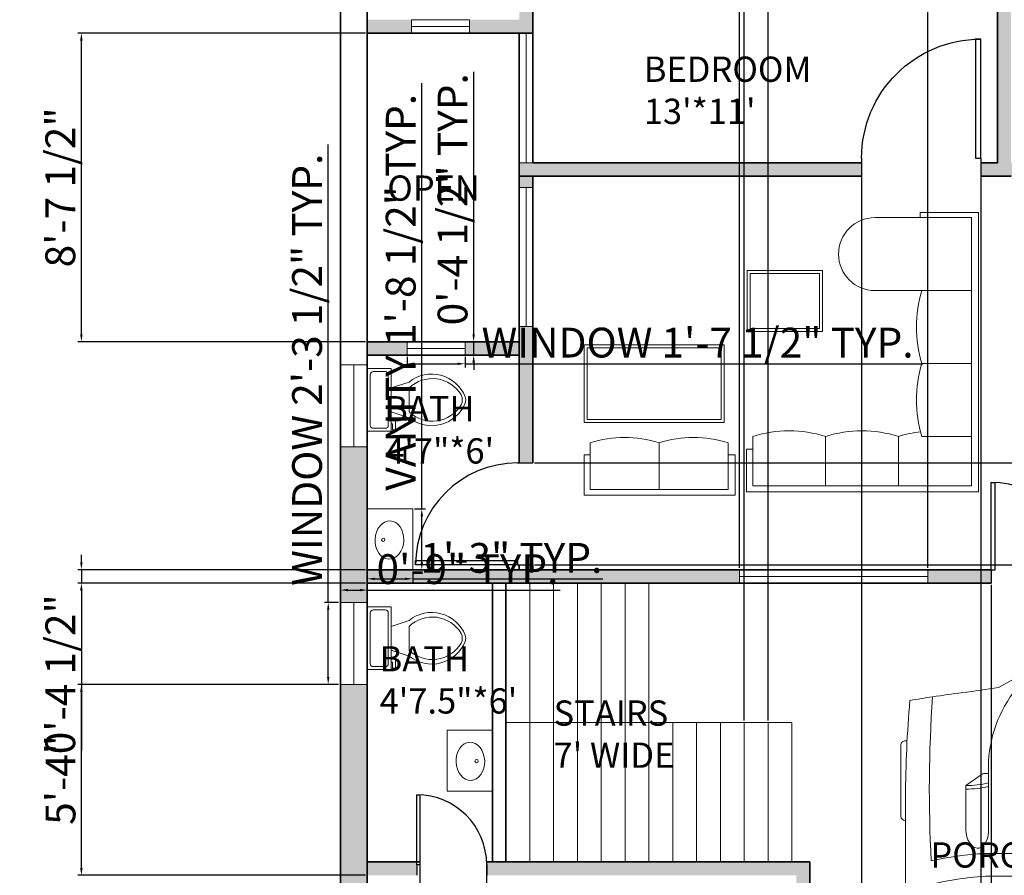
# Model space of a CAD drawing. Units: inches. Extents: x 1698 to 2352, y 1975 to 2732.
# Tile 2 of 4: x 1698 to 2029, y 2234 to 2521. Entities that reach past the tile are written whole.
import ezdxf

# ---------------------------------------------------------------- set-up
doc = ezdxf.new("R2010")
doc.units = ezdxf.units.IN
for name, color, linetype, lineweight in [('A-ANNO-DIMS', 2, 'Continuous', 18), ('A-AREA-IDEN', 7, 'Continuous', 18), ('A-FLOR-FIXT', 231, 'Continuous', 18), ('A-WALL-PATT', 52, 'Continuous', 13), ('car', 171, 'Continuous', 13), ('door', 80, 'Continuous', 25), ('fur', 10, 'Continuous', 18), ('stair', 200, 'Continuous', 18), ('wall', 7, 'Continuous', 35), ('window', 130, 'Continuous', 18)]:
    doc.layers.add(name, color=color, linetype=linetype, lineweight=lineweight)
doc.styles.get("Standard").update_dxf_attribs({"font": 'arial.ttf'})
doc.dimstyles.new('ISO-25', dxfattribs={"dimtxt": 10, "dimasz": 2.5, "dimexe": 1.25, "dimexo": 0.625, "dimtad": 1, "dimdec": 0, "dimlunit": 4, "dimtxsty": 'Standard', "dimcen": 2.5, "dimadec": 0, "dimazin": 0, "dimtfac": 1, "dimtdec": 0, "dimtmove": 0, "dimatfit": 3, "dimfxl": 1, "dimarcsym": 0})

# ---------------------------------------------------------------- blocks, each defined once
blk = doc.blocks.new('*U2')
for p, q in [((0, 0), (0, -6)), ((40, 0), (40, -6))]:
    blk.add_line(p, q)
blk.add_lwpolyline([(0, 0), (0, 40), (1.75, 40), (1.75, 0)], close=True)
blk.add_arc((0, 0), 40, 0, 90)
blk = doc.blocks.new('*U6')
for p, q in [((21.1, 37.41), (21.1, 36.83)), ((46.55, 38.89), (22.35, 38.89)), ((47.8, 37.39), (47.8, 37.41)), ((135.45, 37.07), (135.45, 37.41)), ((136.7, 38.89), (160.9, 38.89)), ((162.15, 37.41), (162.15, 36.77)), ((87.99, 31.87), (74.76, 35.92)), ((134.31, 35.6), (119.29, 31.78)), ((186.47, -33.5), (186.47, 33.5)), ((70.03, 31.54), (86.41, 29.35)), ((188.4, -32.76), (188.4, 32.76)), ((138.42, 29.35), (157.25, 29.35)), ((186.47, 29.35), (167.01, 29.35)), ((164.52, 26.39), (164.52, -26.39)), ((32.27, 11.63), (36.13, 17.17)), ((36.13, 17.17), (50.94, 17.17)), ((32.12, 9.51), (32.12, 11.15)), ((58.92, -10.77), (58.92, 10.77)), ((66.55, -10.53), (66.55, 10.53)), ((186.47, -10.53), (186.47, 10.53)), ((29.77, 9.51), (51.68, 9.51)), ((82.74, 8.5), (82.74, -8.5)), ((3.27, 6.13), (0.1, 0.41)), ((0, 0), (51.68, 0)), ((0.1, -0.41), (3.27, -6.13)), ((29.77, -9.51), (51.68, -9.51)), ((32.12, -9.51), (32.12, -11.15)), ((32.27, -11.63), (36.13, -17.17)), ((36.13, -17.17), (50.94, -17.17)), ((86.41, -29.35), (70.03, -31.54)), ((157.25, -29.35), (138.42, -29.35)), ((167.01, -29.35), (186.47, -29.35)), ((87.99, -31.87), (74.76, -35.92)), ((134.31, -35.6), (119.29, -31.78)), ((21.1, -37.41), (21.1, -36.83)), ((46.55, -38.89), (22.35, -38.89)), ((47.8, -37.39), (47.8, -37.41)), ((135.45, -37.07), (135.45, -37.41)), ((136.7, -38.89), (160.9, -38.89)), ((162.15, -37.41), (162.15, -36.77))]:
    blk.add_line(p, q)
for centre, major_axis, ratio, start_param, end_param in [((41.19, -490.86), (0, 528.23), 0.842304, 0.00281, 0.075598), ((22.35, 37.41), (0, -1.48), 0.842304, 3.141593, 4.712389), ((64.48, -10555.62), (0, 10593.03), 0.842304, -0.013397, 0.002797), ((46.55, 37.41), (0, 1.48), 0.842304, -1.570796, 0), ((136.7, 37.41), (0, -1.48), 0.842304, 3.141593, 4.712389), ((160.9, 37.41), (0, 1.48), 0.842304, -1.570796, 0), ((180.63, 35.84), (0, 2.22), 0.842304, -0.013017, 1.249894), ((64.48, -10556.36), (0, 10595.31), 0.842304, -0.013397, -0.013017), ((183.98, 33.5), (0, -2.96), 0.842304, 1.570796, 3.128196), ((183.98, 32.76), (0, -5.25), 0.842304, 1.570796, 3.128196), ((266.03, -27.52), (0, 313.31), 0.842304, 1.367076, 1.39176), ((64.48, -10555.62), (0, -10591.55), 0.842304, 3.133765, 3.140441), ((135.29, 5.39), (0, 81.77), 0.842304, 1.245306, 1.50788), ((95.79, -3666.35), (0, -3698.24), 0.842304, 3.134049, 3.144098), ((259.18, -27.52), (0, -305.3), 0.842304, 4.528606, 4.561838), ((37.47, -593.96), (0, -623.33), 0.842304, 3.096046, 3.200911), ((134.4, 5.39), (0, -89.78), 0.842304, 4.449482, 4.652344), ((149.6, 2.8), (0, -79.58), 0.842304, 4.372215, 4.640744), ((17.08, 0), (0, 147.02), 0.842304, 4.511394, 4.913384), ((35.91, 0), (0, 147.02), 0.842304, 4.511394, 4.913384), ((167.01, 26.39), (0, 2.96), 0.842304, 0, 1.570796), ((-204.49, 52.4), (0, -250.96), 0.842304, 1.385369, 1.434372), ((13.04, 17.01), (0, 27.42), 0.842304, 4.435146, 4.718221), ((14.2, 17.01), (0, 27.42), 0.842304, 4.435146, 4.718221), ((50.79, 13.34), (6.34, -0.36), 0.603834, -1.395552, 1.581315), ((32.75, 11.15), (0, 0.74), 0.842304, 0.879714, 1.570796), ((29.77, -46.66), (0, 56.17), 0.842304, 0, 0.590319), ((0.62, 0), (0, -0.74), 0.842304, 4.131459, 5.293319), ((29.77, 46.66), (0, 56.17), 0.842304, 2.551274, 3.141593), ((-204.49, -52.4), (0, 250.96), 0.842304, -1.434372, -1.385369), ((13.04, -17.01), (0, -27.42), 0.842304, 1.564964, 1.848039), ((14.2, -17.01), (0, -27.42), 0.842304, 1.564964, 1.848039), ((149.6, -2.8), (0, -79.58), 0.842304, -1.499151, -1.230623), ((32.75, -11.15), (0, -0.74), 0.842304, 4.712389, 5.403472), ((134.4, -5.39), (0, -89.78), 0.842304, -1.510751, -1.307889), ((135.29, -5.39), (0, -81.77), 0.842304, -1.50788, -1.245306), ((259.18, 27.52), (0, 305.3), 0.842304, 1.721348, 1.754579), ((167.01, -26.39), (0, -2.96), 0.842304, 4.712389, 6.283185), ((266.03, 27.52), (0, 313.31), 0.842304, 1.749832, 1.774517), ((37.47, 593.96), (0, -623.33), 0.842304, -0.059319, 0.045547), ((95.79, 3666.35), (0, -3698.24), 0.842304, -0.002505, 0.007544), ((183.98, -32.76), (0, -5.25), 0.842304, 0.013397, 1.570796), ((41.19, 490.86), (0, -528.23), 0.842304, -0.075598, -0.00281), ((64.48, 10555.62), (0, -10591.55), 0.842304, 0.001152, 0.007828), ((183.98, -33.5), (0, 2.96), 0.842304, 3.15499, 4.712389), ((22.35, -37.41), (0, 1.48), 0.842304, 1.570796, 3.141593), ((64.48, 10555.62), (0, 10593.03), 0.842304, 3.138796, 3.15499), ((46.55, -37.41), (0, -1.48), 0.842304, 0, 1.570796), ((136.7, -37.41), (0, -1.48), 0.842304, -1.570796, 0), ((160.9, -37.41), (0, 1.48), 0.842304, 3.141593, 4.712389), ((180.63, -35.84), (0, -2.22), 0.842304, -1.249894, 0.013017), ((64.48, 10556.36), (0, 10595.31), 0.842304, 3.15461, 3.15499)]:
    blk.add_ellipse(centre, major_axis=major_axis, ratio=ratio, start_param=start_param, end_param=end_param)
at = {"extrusion": (0, 0, -1)}
blk.add_ellipse((50.79, -13.34), major_axis=(6.34, 0.36), ratio=0.603834, start_param=-1.395552, end_param=1.581315, dxfattribs=at)
blk = doc.blocks.new('*U4')
for p, q in [((9.5, -6), (9.5, -2)), ((-10, -8.5), (-8, -8.5)), ((-10, -9.5), (-10, -8.5)), ((-7, -9.5), (-10, -9.5)), ((-8, -8.5), (-8, -8)), ((-7, -8), (-7, -9.5)), ((-4, -8), (-6, -14)), ((4, -8), (6, -14)), ((4, -14), (-4, -14))]:
    blk.add_line(p, q)
blk.add_lwpolyline([(10.5, -8), (10.5, 0), (-10.5, 0), (-10.5, -8)], close=True)
for points in [[(-9.5, -2), (-9.5, -6)], [(8.5, -1), (-8.5, -1)], [(-8.5, -7), (8.5, -7)]]:
    blk.add_lwpolyline(points)
for centre, radius, start, end in [((-8.62, -1.88), 0.884, 81.8699, 188.1301), ((8.62, -1.88), 0.884, 351.8699, 98.1301), ((-8.62, -6.12), 0.884, 171.8699, 278.1301), ((8.62, -6.12), 0.884, 261.8699, 8.1301), ((3.52, -21.58), 12.17, 141.4691, 247.9714), ((4.2, -21.82), 11.33, 136.3677, 238.9468), ((-3.52, -21.58), 12.17, 292.0284, 38.5307), ((-4.2, -21.82), 11.33, 301.053, 43.6321), ((0, -27.88), 4, 245.7318, 294.2682), ((0, -29), 4, 254.8605, 285.1395)]:
    blk.add_arc(centre, radius, start, end)
blk = doc.blocks.new('BASIN-VANITY')
blk.add_lwpolyline([(0, 20.39), (15.22, 20.39), (15.22, 0), (0, 0)], close=True)
blk.add_circle((5.32, 10.07), 0.551)
blk.add_ellipse((7.43, 9.98), major_axis=(-0.23, -6.4), ratio=0.75221)
blk = doc.blocks.new('WIN-BATH-19_41')
blk.add_line((0, 2.25), (19.41, 2.25))
blk.add_lwpolyline([(0, 4.5), (19.41, 4.5), (19.41, 0), (0, 0)], close=True)
blk = doc.blocks.new('WIN-BATH-27_526')
blk.add_line((4.5, 27.53), (4.5, 0))
blk.add_lwpolyline([(0, 27.53), (9, 27.53), (9, 0), (0, 0)], close=True)
blk = doc.blocks.new('*D17')
at = {"layer": 'A-ANNO-DIMS', "color": 0, "lineweight": -2, "transparency": 16777216}
for p, q in [((1833.27, 2357.16), (1833.27, 2500.02)), ((1830.84, 2357.16), (1834.52, 2357.16)), ((1833.27, 2339.26), (1833.27, 2354.66)), ((1830.84, 2336.76), (1834.52, 2336.76))]:
    blk.add_line(p, q, dxfattribs=at)
at = {"layer": 'A-ANNO-DIMS', "color": 0, "lineweight": 100, "transparency": 16777216}
for points in [[(1832.85, 2354.66), (1833.69, 2354.66), (1833.27, 2357.16)], [(1832.85, 2339.26), (1833.69, 2339.26), (1833.27, 2336.76)]]:
    blk.add_solid(points, dxfattribs=at)
at = {"layer": 'Defpoints', "color": 0, "lineweight": 100, "transparency": 16777216}
for p in [(1830.21, 2357.16), (1833.27, 2357.16), (1830.21, 2336.76)]:
    blk.add_point(p, dxfattribs=at)
at = {"layer": 'A-ANNO-DIMS', "color": 0, "transparency": 16777216, "insert": (1827.48, 2429.84), "char_height": 10, "attachment_point": 5, "rotation": 90}
blk.add_mtext('VANITY 1\'-8 1/2" TYP.', dxfattribs=at)
blk = doc.blocks.new('*D18')
at = {"layer": 'A-ANNO-DIMS', "color": 0, "lineweight": -2, "transparency": 16777216}
for p, q in [((1814.99, 2336.14), (1814.99, 2332.45)), ((1830.21, 2336.14), (1830.21, 2332.45)), ((1817.49, 2333.7), (1827.71, 2333.7)), ((1830.21, 2333.7), (1893.98, 2333.7))]:
    blk.add_line(p, q, dxfattribs=at)
at = {"layer": 'A-ANNO-DIMS', "color": 0, "lineweight": 100, "transparency": 16777216}
for points in [[(1817.49, 2334.12), (1817.49, 2333.29), (1814.99, 2333.7)], [(1827.71, 2334.12), (1827.71, 2333.29), (1830.21, 2333.7)]]:
    blk.add_solid(points, dxfattribs=at)
at = {"layer": 'Defpoints', "color": 0, "lineweight": 100, "transparency": 16777216}
for p in [(1814.99, 2336.76), (1830.21, 2336.76), (1830.21, 2333.7)]:
    blk.add_point(p, dxfattribs=at)
at = {"layer": 'A-ANNO-DIMS', "color": 0, "transparency": 16777216, "insert": (1863.34, 2339.44), "char_height": 10, "attachment_point": 5}
blk.add_mtext('1\'-3" TYP.', dxfattribs=at)
blk = doc.blocks.new('*D23')
at = {"layer": 'A-ANNO-DIMS', "color": 0, "lineweight": -2, "transparency": 16777216}
for p, q in [((1828.36, 2408.14), (1828.36, 2404.6)), ((1830.86, 2405.85), (1845.27, 2405.85)), ((1847.77, 2408.14), (1847.77, 2404.6)), ((1847.77, 2405.85), (2001.36, 2405.85))]:
    blk.add_line(p, q, dxfattribs=at)
at = {"layer": 'A-ANNO-DIMS', "color": 0, "lineweight": 100, "transparency": 16777216}
for points in [[(1830.86, 2406.27), (1830.86, 2405.43), (1828.36, 2405.85)], [(1845.27, 2406.27), (1845.27, 2405.43), (1847.77, 2405.85)]]:
    blk.add_solid(points, dxfattribs=at)
at = {"layer": 'Defpoints', "color": 0, "lineweight": 100, "transparency": 16777216}
for p in [(1828.36, 2408.76), (1847.77, 2408.76), (1847.77, 2405.85)]:
    blk.add_point(p, dxfattribs=at)
at = {"layer": 'A-ANNO-DIMS', "color": 0, "transparency": 16777216, "insert": (1925.81, 2411.65), "char_height": 10, "attachment_point": 5}
blk.add_mtext('WINDOW 1\'-7 1/2" TYP.', dxfattribs=at)
blk = doc.blocks.new('*D24')
at = {"layer": 'A-ANNO-DIMS', "color": 0, "lineweight": -2, "transparency": 16777216}
for p, q in [((1850.68, 2415.76), (1850.68, 2503.77)), ((1848.39, 2413.26), (1851.93, 2413.26)), ((1850.68, 2408.76), (1850.68, 2413.26)), ((1848.39, 2408.76), (1851.93, 2408.76)), ((1850.68, 2406.26), (1850.68, 2403.76))]:
    blk.add_line(p, q, dxfattribs=at)
at = {"layer": 'A-ANNO-DIMS', "color": 0, "lineweight": 100, "transparency": 16777216}
for points in [[(1850.26, 2415.76), (1851.09, 2415.76), (1850.68, 2413.26)], [(1850.26, 2406.26), (1851.09, 2406.26), (1850.68, 2408.76)]]:
    blk.add_solid(points, dxfattribs=at)
at = {"layer": 'Defpoints', "color": 0, "lineweight": 100, "transparency": 16777216}
for p in [(1847.77, 2413.26), (1850.68, 2413.26), (1847.77, 2408.76)]:
    blk.add_point(p, dxfattribs=at)
at = {"layer": 'A-ANNO-DIMS', "color": 0, "transparency": 16777216, "insert": (1844.88, 2461.02), "char_height": 10, "attachment_point": 5, "rotation": 90}
blk.add_mtext('0\'-4 1/2" TYP.', dxfattribs=at)
blk = doc.blocks.new('*D31')
at = {"layer": 'A-ANNO-DIMS', "color": 0, "lineweight": -2, "transparency": 16777216}
for p, q in [((1801.86, 2325.81), (1801.86, 2479.4)), ((1805.37, 2325.81), (1800.61, 2325.81)), ((1801.86, 2300.78), (1801.86, 2323.31)), ((1805.37, 2298.28), (1800.61, 2298.28))]:
    blk.add_line(p, q, dxfattribs=at)
at = {"layer": 'A-ANNO-DIMS', "color": 0, "lineweight": 100, "transparency": 16777216}
for points in [[(1801.45, 2323.31), (1802.28, 2323.31), (1801.86, 2325.81)], [(1801.45, 2300.78), (1802.28, 2300.78), (1801.86, 2298.28)]]:
    blk.add_solid(points, dxfattribs=at)
at = {"layer": 'Defpoints', "color": 0, "lineweight": 100, "transparency": 16777216}
for p in [(1801.86, 2325.81), (1805.99, 2325.81), (1805.99, 2298.28)]:
    blk.add_point(p, dxfattribs=at)
at = {"layer": 'A-ANNO-DIMS', "color": 0, "transparency": 16777216, "insert": (1796.06, 2403.85), "char_height": 10, "attachment_point": 5, "rotation": 90}
blk.add_mtext('WINDOW 2\'-3 1/2" TYP.', dxfattribs=at)
blk = doc.blocks.new('*D32')
at = {"layer": 'A-ANNO-DIMS', "color": 0, "lineweight": -2, "transparency": 16777216}
for p, q in [((1805.99, 2326.43), (1805.99, 2331.18)), ((1808.49, 2329.93), (1812.49, 2329.93)), ((1814.99, 2326.43), (1814.99, 2331.18)), ((1814.99, 2329.93), (1879.7, 2329.93))]:
    blk.add_line(p, q, dxfattribs=at)
at = {"layer": 'A-ANNO-DIMS', "color": 0, "lineweight": 100, "transparency": 16777216}
for points in [[(1808.49, 2330.35), (1808.49, 2329.52), (1805.99, 2329.93)], [(1812.49, 2330.35), (1812.49, 2329.52), (1814.99, 2329.93)]]:
    blk.add_solid(points, dxfattribs=at)
at = {"layer": 'Defpoints', "color": 0, "lineweight": 100, "transparency": 16777216}
for p in [(1814.99, 2329.93), (1805.99, 2325.81), (1814.99, 2325.81)]:
    blk.add_point(p, dxfattribs=at)
at = {"layer": 'A-ANNO-DIMS', "color": 0, "transparency": 16777216, "insert": (1848.59, 2335.67), "char_height": 10, "attachment_point": 5}
blk.add_mtext('0\'-9" TYP.', dxfattribs=at)
blk = doc.blocks.new('*D35')
at = {"layer": 'A-ANNO-DIMS', "color": 0, "lineweight": -2, "transparency": 16777216}
for p, q in [((1832.59, 2238.14), (1832.59, 1983.28)), ((1855.03, 2238.14), (1855.03, 1983.28)), ((1835.09, 1984.53), (1852.53, 1984.53)), ((1855.03, 1984.53), (1915.49, 1984.53))]:
    blk.add_line(p, q, dxfattribs=at)
at = {"layer": 'A-ANNO-DIMS', "color": 0, "lineweight": 100, "transparency": 16777216}
for points in [[(1835.09, 1984.94), (1835.09, 1984.11), (1832.59, 1984.53)], [(1852.53, 1984.94), (1852.53, 1984.11), (1855.03, 1984.53)]]:
    blk.add_solid(points, dxfattribs=at)
at = {"layer": 'Defpoints', "color": 0, "lineweight": 100, "transparency": 16777216}
for p in [(1832.59, 2238.76), (1855.03, 2238.76), (1855.03, 1984.53)]:
    blk.add_point(p, dxfattribs=at)
at = {"layer": 'A-ANNO-DIMS', "color": 0, "transparency": 16777216, "insert": (1886.51, 1990.32), "char_height": 10, "attachment_point": 5}
blk.add_mtext('1\'-10 1/2"', dxfattribs=at)
blk = doc.blocks.new('*D36')
at = {"layer": 'A-ANNO-DIMS', "color": 0, "lineweight": -2, "transparency": 16777216}
for p, q in [((1941.49, 2286.14), (1941.49, 2651.46)), ((1943.99, 2650.21), (1946.99, 2650.21)), ((1949.49, 2286.14), (1949.49, 2651.46)), ((1949.49, 2650.21), (1979.82, 2650.21))]:
    blk.add_line(p, q, dxfattribs=at)
at = {"layer": 'A-ANNO-DIMS', "color": 0, "lineweight": 100, "transparency": 16777216}
for points in [[(1943.99, 2650.63), (1943.99, 2649.8), (1941.49, 2650.21)], [(1946.99, 2650.63), (1946.99, 2649.8), (1949.49, 2650.21)]]:
    blk.add_solid(points, dxfattribs=at)
at = {"layer": 'Defpoints', "color": 0, "lineweight": 100, "transparency": 16777216}
for p in [(1949.49, 2650.21), (1941.49, 2285.51), (1949.49, 2285.51)]:
    blk.add_point(p, dxfattribs=at)
at = {"layer": 'A-ANNO-DIMS', "color": 0, "transparency": 16777216, "insert": (1965.91, 2655.94), "char_height": 10, "attachment_point": 5}
blk.add_mtext('0\'-8"', dxfattribs=at)
blk = doc.blocks.new('*D37')
at = {"layer": 'A-ANNO-DIMS', "color": 0, "lineweight": -2, "transparency": 16777216}
for p, q in [((2024.3, 2331.64), (2024.3, 1983.28)), ((2083.04, 2331.64), (2083.04, 1983.28)), ((2026.8, 1984.53), (2080.54, 1984.53)), ((2083.04, 1984.53), (2144.84, 1984.53))]:
    blk.add_line(p, q, dxfattribs=at)
at = {"layer": 'A-ANNO-DIMS', "color": 0, "lineweight": 100, "transparency": 16777216}
for points in [[(2026.8, 1984.94), (2026.8, 1984.11), (2024.3, 1984.53)], [(2080.54, 1984.94), (2080.54, 1984.11), (2083.04, 1984.53)]]:
    blk.add_solid(points, dxfattribs=at)
at = {"layer": 'Defpoints', "color": 0, "lineweight": 100, "transparency": 16777216}
for p in [(2024.3, 2332.26), (2083.04, 2332.26), (2083.04, 1984.53)]:
    blk.add_point(p, dxfattribs=at)
at = {"layer": 'A-ANNO-DIMS', "color": 0, "transparency": 16777216, "insert": (2115.19, 1990.32), "char_height": 10, "attachment_point": 5}
blk.add_mtext('4\'-10 1/2"', dxfattribs=at)
blk = doc.blocks.new('*D39')
at = {"layer": 'A-ANNO-DIMS', "color": 0, "lineweight": -2, "transparency": 16777216}
for p, q in [((1980.85, 2472.64), (1980.85, 1983.28)), ((2020.85, 2472.64), (2020.85, 1983.28)), ((1983.35, 1984.53), (2018.35, 1984.53))]:
    blk.add_line(p, q, dxfattribs=at)
at = {"layer": 'A-ANNO-DIMS', "color": 0, "lineweight": 100, "transparency": 16777216}
for points in [[(1983.35, 1984.94), (1983.35, 1984.11), (1980.85, 1984.53)], [(2018.35, 1984.94), (2018.35, 1984.11), (2020.85, 1984.53)]]:
    blk.add_solid(points, dxfattribs=at)
at = {"layer": 'Defpoints', "color": 0, "lineweight": 100, "transparency": 16777216}
for p in [(1980.85, 2473.26), (2020.85, 2473.26), (2020.85, 1984.53)]:
    blk.add_point(p, dxfattribs=at)
at = {"layer": 'A-ANNO-DIMS', "color": 0, "transparency": 16777216, "insert": (2000.85, 1990.26), "char_height": 10, "attachment_point": 5}
blk.add_mtext('3\'-4"', dxfattribs=at)
blk = doc.blocks.new('*D42')
at = {"layer": 'A-ANNO-DIMS', "color": 0, "lineweight": -2, "transparency": 16777216}
for p, q in [((1805.37, 2298.28), (1717.79, 2298.28)), ((1719.04, 2236.76), (1719.04, 2295.78)), ((1814.37, 2234.26), (1717.79, 2234.26))]:
    blk.add_line(p, q, dxfattribs=at)
at = {"layer": 'A-ANNO-DIMS', "color": 0, "lineweight": 100, "transparency": 16777216}
for points in [[(1718.62, 2295.78), (1719.46, 2295.78), (1719.04, 2298.28)], [(1718.62, 2236.76), (1719.46, 2236.76), (1719.04, 2234.26)]]:
    blk.add_solid(points, dxfattribs=at)
at = {"layer": 'Defpoints', "color": 0, "lineweight": 100, "transparency": 16777216}
for p in [(1719.04, 2298.28), (1805.99, 2298.28), (1814.99, 2234.26)]:
    blk.add_point(p, dxfattribs=at)
at = {"layer": 'A-ANNO-DIMS', "color": 0, "transparency": 16777216, "insert": (1713.33, 2266.27), "char_height": 10, "attachment_point": 5, "rotation": 90}
blk.add_mtext('5\'-4"', dxfattribs=at)
blk = doc.blocks.new('*D44')
at = {"layer": 'A-ANNO-DIMS', "color": 0, "lineweight": -2, "transparency": 16777216}
for p, q in [((1719.04, 2339.26), (1719.04, 2341.76)), ((1814.37, 2336.76), (1717.79, 2336.76)), ((1719.04, 2336.76), (1719.04, 2332.26)), ((1814.37, 2332.26), (1717.79, 2332.26)), ((1719.04, 2329.76), (1719.04, 2276.13))]:
    blk.add_line(p, q, dxfattribs=at)
at = {"layer": 'A-ANNO-DIMS', "color": 0, "lineweight": 100, "transparency": 16777216}
for points in [[(1718.62, 2339.26), (1719.46, 2339.26), (1719.04, 2336.76)], [(1718.62, 2329.76), (1719.46, 2329.76), (1719.04, 2332.26)]]:
    blk.add_solid(points, dxfattribs=at)
at = {"layer": 'Defpoints', "color": 0, "lineweight": 100, "transparency": 16777216}
for p in [(1814.99, 2336.76), (1719.04, 2332.26), (1814.99, 2332.26)]:
    blk.add_point(p, dxfattribs=at)
at = {"layer": 'A-ANNO-DIMS', "color": 0, "transparency": 16777216, "insert": (1713.25, 2301.7), "char_height": 10, "attachment_point": 5, "rotation": 90}
blk.add_mtext('0\'-4 1/2"', dxfattribs=at)
blk = doc.blocks.new('*D45')
at = {"layer": 'A-ANNO-DIMS', "color": 0, "lineweight": -2, "transparency": 16777216}
for p, q in [((2342.94, 2372.57), (2342.94, 2410.85)), ((1871.12, 2372.57), (2344.19, 2372.57)), ((2342.94, 2340.87), (2342.94, 2370.07)), ((1871.12, 2338.37), (2344.19, 2338.37))]:
    blk.add_line(p, q, dxfattribs=at)
at = {"layer": 'A-ANNO-DIMS', "color": 0, "lineweight": 100, "transparency": 16777216}
for points in [[(2342.52, 2370.07), (2343.36, 2370.07), (2342.94, 2372.57)], [(2342.52, 2340.87), (2343.36, 2340.87), (2342.94, 2338.37)]]:
    blk.add_solid(points, dxfattribs=at)
at = {"layer": 'Defpoints', "color": 0, "lineweight": 100, "transparency": 16777216}
for p in [(1870.49, 2372.57), (2342.94, 2372.57), (1870.49, 2338.37)]:
    blk.add_point(p, dxfattribs=at)
at = {"layer": 'A-ANNO-DIMS', "color": 0, "transparency": 16777216, "insert": (2337.21, 2392.96), "char_height": 10, "attachment_point": 5, "rotation": 90}
blk.add_mtext('2\'-10"', dxfattribs=at)
blk = doc.blocks.new('*D46')
at = {"layer": 'A-ANNO-DIMS', "color": 0, "lineweight": -2, "transparency": 16777216}
for p, q in [((1814.37, 2516.76), (1717.79, 2516.76)), ((1719.04, 2415.76), (1719.04, 2514.26)), ((1814.37, 2413.26), (1717.79, 2413.26))]:
    blk.add_line(p, q, dxfattribs=at)
at = {"layer": 'A-ANNO-DIMS', "color": 0, "lineweight": 100, "transparency": 16777216}
for points in [[(1718.62, 2514.26), (1719.46, 2514.26), (1719.04, 2516.76)], [(1718.62, 2415.76), (1719.46, 2415.76), (1719.04, 2413.26)]]:
    blk.add_solid(points, dxfattribs=at)
at = {"layer": 'Defpoints', "color": 0, "lineweight": 100, "transparency": 16777216}
for p in [(1719.04, 2516.76), (1814.99, 2516.76), (1814.99, 2413.26)]:
    blk.add_point(p, dxfattribs=at)
at = {"layer": 'A-ANNO-DIMS', "color": 0, "transparency": 16777216, "insert": (1713.25, 2465.01), "char_height": 10, "attachment_point": 5, "rotation": 90}
blk.add_mtext('8\'-7 1/2"', dxfattribs=at)
blk = doc.blocks.new('*D50')
at = {"layer": 'A-ANNO-DIMS', "color": 0, "lineweight": -2, "transparency": 16777216}
for p, q in [((1939.87, 2337.39), (1939.87, 2651.46)), ((1942.37, 2650.21), (2000.54, 2650.21)), ((2003.04, 2337.39), (2003.04, 2651.46))]:
    blk.add_line(p, q, dxfattribs=at)
at = {"layer": 'A-ANNO-DIMS', "color": 0, "lineweight": 100, "transparency": 16777216}
for points in [[(1942.37, 2650.63), (1942.37, 2649.8), (1939.87, 2650.21)], [(2000.54, 2650.63), (2000.54, 2649.8), (2003.04, 2650.21)]]:
    blk.add_solid(points, dxfattribs=at)
at = {"layer": 'Defpoints', "color": 0, "lineweight": 100, "transparency": 16777216}
for p in [(2003.04, 2650.21), (1939.87, 2336.76), (2003.04, 2336.76)]:
    blk.add_point(p, dxfattribs=at)
at = {"layer": 'A-ANNO-DIMS', "color": 0, "transparency": 16777216, "insert": (1971.45, 2655.95), "char_height": 10, "attachment_point": 5}
blk.add_mtext('5\'-3"', dxfattribs=at)

msp = doc.modelspace()

# ---------------------------------------------------------------- hatches: boundary and pattern name
at = {"layer": 'A-WALL-PATT'}
h = msp.add_hatch(color=256, dxfattribs=at)
h.dxf.hatch_style = 1
h.paths.add_polyline_path([(1910.52, 2614.26), (1805.99, 2614.26), (1805.99, 2549.47), (1814.99, 2549.47), (1814.99, 2605.26), (1910.52, 2605.26)])
h.paths.add_polyline_path([(2084.19, 2614.26), (1972.89, 2614.26), (1972.89, 2605.26), (2026.49, 2605.26), (2084.19, 2605.26)])
h.paths.add_polyline_path([(2255.99, 2614.26), (2146.56, 2614.26), (2146.56, 2605.26), (2148.21, 2605.26), (2186.99, 2605.26), (2246.99, 2605.26), (2246.99, 2546.53), (2255.99, 2546.53)])
h.paths.add_polyline_path([(2191.49, 2605.26), (2186.99, 2605.26), (2186.99, 2595.02), (2191.49, 2595.02)], flags=17)
h.paths.add_polyline_path([(2191.49, 2563.28), (2186.99, 2563.28), (2186.99, 2510.76), (2191.49, 2510.76)])
h.paths.add_polyline_path([(2246.99, 2515.26), (2191.49, 2515.26), (2191.49, 2510.76), (2246.99, 2510.76)])
h.paths.add_polyline_path([(2030.99, 2605.26), (2026.49, 2605.26), (2026.49, 2473.26), (2020.85, 2473.26), (2020.85, 2468.76), (2030.99, 2468.76)])
h.paths.add_polyline_path([(1980.85, 2473.26), (1870.49, 2473.26), (1865.99, 2473.26), (1865.99, 2468.76), (1980.85, 2468.76)])
h.paths.add_polyline_path([(1828.36, 2413.26), (1814.99, 2413.26), (1814.99, 2408.76), (1828.36, 2408.76)])
h.paths.add_polyline_path([(1865.99, 2413.26), (1847.77, 2413.26), (1847.77, 2408.76), (1865.99, 2408.76)])
h.paths.add_polyline_path([(1870.49, 2418.36), (1865.99, 2418.36), (1865.99, 2372.57), (1870.49, 2372.57)])
h.paths.add_polyline_path([(2036.32, 2473.26), (2030.99, 2473.26), (2030.99, 2468.76), (2036.32, 2468.76)])
h.paths.add_polyline_path([(2191.49, 2473.26), (2186.99, 2473.26), (2076.32, 2473.26), (2076.32, 2468.76), (2191.49, 2468.76)])
h.paths.add_polyline_path([(2246.99, 2471.76), (2191.49, 2471.76), (2191.49, 2468.76), (2246.99, 2468.76)])
h.paths.add_polyline_path([(2255.99, 2406.37), (2246.99, 2406.37), (2246.99, 2404.25), (2246.99, 2336.76), (2246.99, 2083.26), (2127.92, 2083.26), (2127.92, 2074.26), (2255.99, 2074.26)])
h.paths.add_polyline_path([(2110.49, 2336.76), (2083.04, 2336.76), (2083.04, 2336.67), (2083.04, 2332.26), (2110.49, 2332.26)])
h.paths.add_polyline_path([(2024.3, 2336.76), (2003.04, 2336.76), (2003.04, 2332.26), (2024.3, 2332.26)])
h.paths.add_polyline_path([(2246.99, 2164.26), (2216.76, 2164.26), (2216.76, 2155.26), (2246.99, 2155.26)], flags=17)
h.paths.add_polyline_path([(1958.99, 2083.26), (1927.89, 2083.26), (1927.89, 2074.26), (1958.99, 2074.26)])
h.paths.add_polyline_path([(1963.49, 2185.34), (1958.99, 2185.34), (1958.99, 2083.26), (1963.49, 2083.26)])
h.paths.add_polyline_path([(1963.49, 2238.76), (1855.03, 2238.76, -0.010403), (1855.05, 2237.79), (1855.05, 2234.26), (1958.99, 2234.26), (1958.99, 2225.34), (1963.49, 2225.34)])
h.paths.add_polyline_path([(1831.56, 2237.79), (1831.56, 2238.76), (1814.99, 2238.76), (1814.99, 2234.26), (1831.56, 2234.26)])
h.paths.add_polyline_path([(1939.87, 2336.76), (1814.99, 2336.76), (1814.99, 2332.26), (1856.99, 2332.26), (1939.87, 2332.26)])
h.paths.add_polyline_path([(1814.99, 2377.93), (1805.99, 2377.93), (1805.99, 2325.81), (1814.99, 2325.81)])
h.paths.add_polyline_path([(1829.84, 2521.26), (1814.99, 2521.26), (1814.99, 2516.76), (1829.84, 2516.76)])
h.paths.add_polyline_path([(2255.99, 2471.76), (2246.99, 2471.76), (2246.99, 2438.09), (2255.99, 2438.09)])
h = msp.add_hatch(color=256, dxfattribs=at)
h.dxf.hatch_style = 1
h.paths.add_polyline_path([(1870.49, 2565.42), (1865.99, 2565.42), (1865.99, 2521.26), (1849.25, 2521.26), (1849.25, 2516.76), (1870.49, 2516.76)])
h.paths.add_polyline_path([(1870.49, 2605.26), (1865.99, 2605.26), (1865.99, 2598.8), (1870.49, 2598.8)])
h.paths.add_polyline_path([(2246.99, 2336.76), (2147.99, 2336.76), (2147.99, 2360.76), (2147.99, 2418.65), (2143.49, 2418.65), (2143.49, 2332.26), (2246.99, 2332.26)])
h.paths.add_polyline_path([(2143.49, 2336.76), (2110.49, 2336.76), (2110.49, 2325.07), (2114.99, 2325.07), (2114.99, 2332.26), (2143.49, 2332.26)])
h.paths.add_polyline_path([(2114.99, 2285.07), (2110.49, 2285.07), (2110.49, 2155.26), (2141.76, 2155.26), (2141.76, 2164.26), (2114.99, 2164.26)])
h.paths.add_polyline_path([(1814.99, 2298.28), (1805.99, 2298.28), (1805.99, 2074.26), (1852.89, 2074.26), (1852.89, 2083.26), (1814.99, 2083.26)])
h = msp.add_hatch(color=256, dxfattribs=at)
h.dxf.hatch_style = 1
h.paths.add_polyline_path([(1870.49, 2468.76), (1865.99, 2468.76), (1865.99, 2464.98), (1870.49, 2464.98)])

# ---------------------------------------------------------------- linework, layer by layer
at = {"layer": 'fur'}
for p, q in [((2020.07, 2456.59), (2000.5, 2456.59)), ((2000.5, 2456.59), (2000.5, 2454.86)), ((2020.07, 2377.16), (2020.07, 2456.59)), ((1985.35, 2454.86), (2001.1, 2454.86)), ((2017.68, 2454.86), (2001.1, 2454.86)), ((2017.68, 2430.4), (2017.68, 2454.86)), ((2001.1, 2430.4), (1985.35, 2430.4)), ((2017.68, 2430.4), (2001.1, 2430.4)), ((2001.1, 2430.4), (2017.68, 2430.4)), ((2017.68, 2405.94), (2017.68, 2430.4)), ((2017.68, 2405.94), (2001.1, 2405.94)), ((2001.1, 2405.94), (2017.68, 2405.94)), ((2017.68, 2381.48), (2017.68, 2405.94)), ((1912.9, 2379.34), (1912.9, 2363.66)), ((1968.77, 2381.48), (1968.77, 2364.9)), ((1968.77, 2381.48), (1968.77, 2364.9)), ((1993.23, 2364.9), (1993.23, 2381.48)), ((1993.23, 2381.48), (1993.23, 2364.9)), ((2001.1, 2381.48), (2017.68, 2381.48)), ((2017.68, 2364.9), (2017.68, 2381.48)), ((1944.31, 2377.16), (1942.24, 2377.16)), ((1942.24, 2377.16), (1942.24, 2362.91)), ((1944.31, 2377.16), (1944.31, 2377.16)), ((2020.07, 2362.91), (2020.07, 2377.16)), ((1889.75, 2375.26), (1887.8, 2375.26)), ((1887.8, 2375.26), (1887.8, 2361.77)), ((1889.75, 2375.26), (1889.75, 2375.26)), ((1938.41, 2375.26), (1936.04, 2375.26)), ((1938.41, 2361.77), (1938.41, 2375.26)), ((1942.24, 2362.91), (1995.74, 2362.91)), ((1968.77, 2364.9), (1993.23, 2364.9)), ((1993.23, 2364.9), (2017.68, 2364.9)), ((1995.74, 2362.91), (2020.07, 2362.91)), ((1887.8, 2361.77), (1938.41, 2361.77))]:
    msp.add_line(p, q, dxfattribs=at)
for points in [[(1942.41, 2437.12), (1967.78, 2437.12), (1967.78, 2416.66), (1942.41, 2416.66)], [(1943.41, 2436.12), (1966.78, 2436.12), (1966.78, 2417.66), (1943.41, 2417.66)], [(1887.74, 2386.16), (1934.69, 2386.16), (1934.69, 2412.22), (1887.74, 2412.22)], [(1888.74, 2387.16), (1933.69, 2387.16), (1933.69, 2411.22), (1888.74, 2411.22)]]:
    msp.add_lwpolyline(points, close=True, dxfattribs=at)
for points in [[(1936.04, 2379.34), (1936.04, 2363.66), (1889.75, 2363.66), (1889.75, 2379.34)], [(1993.23, 2381.48), (1993.23, 2364.9), (1944.31, 2364.9), (1944.31, 2381.48)]]:
    msp.add_lwpolyline(points, dxfattribs=at)
for centre, radius, start, end in [((1985.35, 2442.63), 12.23, 90, 270), ((2040.26, 2418.17), 41.02, 162.6553, 197.3447), ((2040.26, 2393.71), 41.02, 162.6553, 197.3447), ((1956.54, 2342.32), 41.02, 72.6553, 107.3447), ((1981, 2342.32), 41.02, 72.6553, 107.3447), ((1981, 2342.32), 41.02, 72.6553, 107.3447), ((2005.45, 2342.32), 41.02, 96.7335, 107.3447), ((1901.32, 2342.3), 38.81, 72.6553, 107.3447), ((1924.47, 2342.3), 38.81, 72.6553, 107.3447)]:
    msp.add_arc(centre, radius, start, end, dxfattribs=at)
at = {"layer": 'stair'}
for p, q in [((1861.49, 2285.51), (1861.49, 2332.26)), ((1869.49, 2332.26), (1869.49, 2238.76)), ((1877.49, 2332.26), (1877.49, 2238.76)), ((1885.49, 2332.26), (1885.49, 2238.76)), ((1893.49, 2332.26), (1893.49, 2238.76)), ((1901.49, 2332.26), (1901.49, 2238.76)), ((1909.49, 2332.26), (1909.49, 2238.76)), ((1861.49, 2285.51), (1956.82, 2285.51)), ((1917.49, 2285.51), (1917.49, 2238.76)), ((1925.49, 2285.51), (1925.49, 2238.76)), ((1933.49, 2285.51), (1933.49, 2238.76)), ((1941.49, 2285.51), (1941.49, 2238.76)), ((1949.49, 2285.51), (1949.49, 2238.76)), ((1957.49, 2285.51), (1956.82, 2285.51)), ((1957.49, 2285.51), (1957.49, 2238.76))]:
    msp.add_line(p, q, dxfattribs=at)
at = {"layer": 'wall'}
for p, q in [((2026.49, 2605.26), (2026.49, 2473.26)), ((1870.49, 2516.76), (1870.49, 2565.42)), ((1814.99, 2516.76), (1870.49, 2516.76)), ((1814.99, 2516.76), (1814.99, 2416.96)), ((1865.99, 2468.76), (1865.99, 2516.76)), ((1870.49, 2473.26), (1870.49, 2516.76)), ((1980.85, 2473.26), (1870.49, 2473.26)), ((2026.49, 2473.26), (2020.85, 2473.26)), ((1865.99, 2468.76), (1865.99, 2372.57)), ((1980.85, 2468.76), (1865.99, 2468.76)), ((1870.49, 2468.76), (1870.49, 2372.57)), ((2030.99, 2468.76), (2020.85, 2468.76)), ((1814.99, 2416.96), (1814.99, 2413.26)), ((1814.99, 2413.26), (1865.99, 2413.26)), ((1814.99, 2336.76), (1814.99, 2408.76)), ((1814.99, 2408.76), (1865.99, 2408.76)), ((2003.04, 2336.76), (1814.99, 2336.76)), ((1865.99, 2338.37), (1865.99, 2336.76)), ((1870.49, 2338.37), (1870.49, 2336.76)), ((2003.04, 2336.76), (2024.3, 2336.76)), ((1814.99, 2332.26), (1856.99, 2332.26)), ((2003.04, 2332.26), (1814.99, 2332.26)), ((1856.99, 2332.26), (1856.99, 2238.76)), ((1861.49, 2332.26), (1861.49, 2238.76)), ((2003.04, 2332.26), (2024.3, 2332.26)), ((1832.59, 2238.76), (1814.99, 2238.76)), ((1963.49, 2238.76), (1855.03, 2238.76)), ((1963.49, 2225.34), (1963.49, 2238.76))]:
    msp.add_line(p, q, dxfattribs=at)
for points in [[(2127.92, 2074.26), (2255.99, 2074.26), (2255.99, 2614.26), (1805.99, 2614.26), (1805.99, 2074.26), (1958.99, 2074.26)], [(2127.92, 2083.26), (2246.99, 2083.26), (2246.99, 2605.26), (1814.99, 2605.26), (1814.99, 2516.76)], [(1814.99, 2413.26), (1814.99, 2083.26), (1976.89, 2083.26)]]:
    msp.add_lwpolyline(points, dxfattribs=at)
at = {"layer": 'window'}
for p, q in [((1868.24, 2516.76), (1868.24, 2473.26)), ((1868.24, 2418.36), (1868.24, 2464.98)), ((1939.87, 2334.51), (2003.04, 2334.51))]:
    msp.add_line(p, q, dxfattribs=at)
for points in [[(1865.99, 2516.76), (1870.49, 2516.76), (1870.49, 2473.26), (1865.99, 2473.26)], [(1865.99, 2418.36), (1870.49, 2418.36), (1870.49, 2464.98), (1865.99, 2464.98)], [(1939.87, 2336.76), (2003.04, 2336.76), (2003.04, 2332.26), (1939.87, 2332.26)]]:
    msp.add_lwpolyline(points, close=True, dxfattribs=at)

# ---------------------------------------------------------------- block references
at = {"layer": 'A-FLOR-FIXT', "rotation": 90}
for p in [(1814.99, 2393.73), (1814.99, 2313.77)]:
    msp.add_blockref('*U4', p, dxfattribs=at)
at = {"layer": 'A-FLOR-FIXT'}
msp.add_blockref('BASIN-VANITY', (1814.99, 2336.76), dxfattribs=at)
at = {"layer": 'A-FLOR-FIXT', "extrusion": (0, 0, -1), "zscale": -1}
msp.add_blockref('BASIN-VANITY', (-1856.99, 2262.5), dxfattribs=at)
at = {"layer": 'car', "rotation": 270}
msp.add_blockref('*U6', (2032.95, 2300.49), dxfattribs=at)
at = {"layer": 'door', "xscale": -1}
msp.add_blockref('*U2', (2020.85, 2474.76), dxfattribs=at)
at = {"layer": 'door', "xscale": 0.8550076532473024, "yscale": 0.8550076532473024, "zscale": 0.8550076532473024, "rotation": 90}
msp.add_blockref('*U2', (1865.36, 2338.37), dxfattribs=at)
at = {"layer": 'door'}
for p, xscale, yscale, zscale in [((2024.3, 2336.67), 0.734231061655472, 0.734231061655472, 0.734231061655472), ((1831.56, 2237.79), 0.5871648489528541, 0.5871648489528541, 0.5871648489528541)]:
    msp.add_blockref('*U2', p, dxfattribs=dict(at, xscale=xscale, yscale=yscale, zscale=zscale))
at = {"layer": 'window'}
for name, p in [('WIN-BATH-19_41', (1829.84, 2516.76)), ('WIN-BATH-19_41', (1828.36, 2408.76)), ('WIN-BATH-27_526', (1805.99, 2377.93)), ('WIN-BATH-27_526', (1805.99, 2298.28))]:
    msp.add_blockref(name, p, dxfattribs=at)

# ---------------------------------------------------------------- texts
at = {"layer": 'A-AREA-IDEN', "char_height": 8.476, "attachment_point": 1}
for s, insert in [("BEDROOM\\P13'*11'", (1907.78, 2508.89)), ('OPEN', (1821.69, 2469.01)), ('BATH\\P4\'7"*6\'', (1820.98, 2394.99)), ('BATH\\P4\'7.5"*6\'', (1819.12, 2311.12)), ("STAIRS\\P7' WIDE", (1877.49, 2292.92)), ('PORCH\\P11\'6"*20\'', (2003.94, 2245.32))]:
    msp.add_mtext_dynamic_manual_height_columns(s, width=272.6258, gutter_width=42.38, heights=[0], dxfattribs=dict(at, insert=insert))

# ---------------------------------------------------------------- dimensions: what is measured, and where the dimension line sits
at = {"layer": 'A-ANNO-DIMS'}
for base, p1, p2, picture, middle in [((2003.04, 2650.21), (1939.87, 2336.76), (2003.04, 2336.76), '*D50', (1971.45, 2655.95)), ((1949.49, 2650.21), (1941.49, 2285.51), (1949.49, 2285.51), '*D36', (1965.91, 2655.94)), ((2020.85, 1984.53), (1980.85, 2473.26), (2020.85, 2473.26), '*D39', (2000.85, 1990.26)), ((2083.04, 1984.53), (2024.3, 2332.26), (2083.04, 2332.26), '*D37', (2115.19, 1990.32)), ((1855.03, 1984.53), (1832.59, 2238.76), (1855.03, 2238.76), '*D35', (1886.51, 1990.32))]:
    dim = msp.add_linear_dim(base=base, p1=p1, p2=p2, dimstyle='ISO-25', override={"dimdec": 1, "dimlfac": 1, "dimrnd": 0, "dimzin": 1, "dimdsep": 46, "dimlunit": 4, "dimfrac": 2}, dxfattribs=at)
    dim.commit()
    dim.dimension.update_dxf_attribs({"geometry": picture, "text_midpoint": middle})
for base, p1, p2, picture, middle in [((1719.04, 2516.76), (1814.99, 2413.26), (1814.99, 2516.76), '*D46', (1713.25, 2465.01)), ((2342.94, 2372.57), (1870.49, 2338.37), (1870.49, 2372.57), '*D45', (2337.21, 2392.96)), ((1719.04, 2332.26), (1814.99, 2336.76), (1814.99, 2332.26), '*D44', (1713.25, 2301.7)), ((1719.04, 2298.28), (1814.99, 2234.26), (1805.99, 2298.28), '*D42', (1713.33, 2266.27))]:
    dim = msp.add_linear_dim(base=base, p1=p1, p2=p2, angle=90, dimstyle='ISO-25', override={"dimdec": 1, "dimlfac": 1, "dimrnd": 0, "dimzin": 1, "dimdsep": 46, "dimlunit": 4, "dimfrac": 2}, dxfattribs=at)
    dim.commit()
    dim.dimension.update_dxf_attribs({"geometry": picture, "text_midpoint": middle})
for base, p1, p2, text, picture, middle in [((1850.68, 2413.26), (1847.77, 2408.76), (1847.77, 2413.26), '<> TYP.', '*D24', (1844.88, 2461.02)), ((1833.27, 2357.16), (1830.21, 2336.76), (1830.21, 2357.16), 'VANITY <> TYP.', '*D17', (1827.48, 2429.84)), ((1801.86, 2325.81), (1805.99, 2298.28), (1805.99, 2325.81), 'WINDOW <> TYP.', '*D31', (1796.06, 2403.85))]:
    dim = msp.add_linear_dim(base=base, p1=p1, p2=p2, angle=90, text=text, dimstyle='ISO-25', override={"dimdec": 1, "dimlfac": 1, "dimrnd": 0, "dimzin": 1, "dimdsep": 46, "dimlunit": 4, "dimfrac": 2}, dxfattribs=at)
    dim.commit()
    dim.dimension.update_dxf_attribs({"geometry": picture, "text_midpoint": middle})
for base, p1, p2, text, picture, middle in [((1847.77, 2405.85), (1828.36, 2408.76), (1847.77, 2408.76), 'WINDOW <> TYP.', '*D23', (1925.81, 2411.65)), ((1830.21, 2333.7), (1814.99, 2336.76), (1830.21, 2336.76), '<> TYP.', '*D18', (1863.34, 2339.44)), ((1814.99, 2329.93), (1805.99, 2325.81), (1814.99, 2325.81), '<> TYP.', '*D32', (1848.59, 2335.67))]:
    dim = msp.add_linear_dim(base=base, p1=p1, p2=p2, text=text, dimstyle='ISO-25', override={"dimdec": 1, "dimlfac": 1, "dimrnd": 0, "dimzin": 1, "dimdsep": 46, "dimlunit": 4, "dimfrac": 2}, dxfattribs=at)
    dim.commit()
    dim.dimension.update_dxf_attribs({"geometry": picture, "text_midpoint": middle})

doc.saveas('drawing.dxf')
